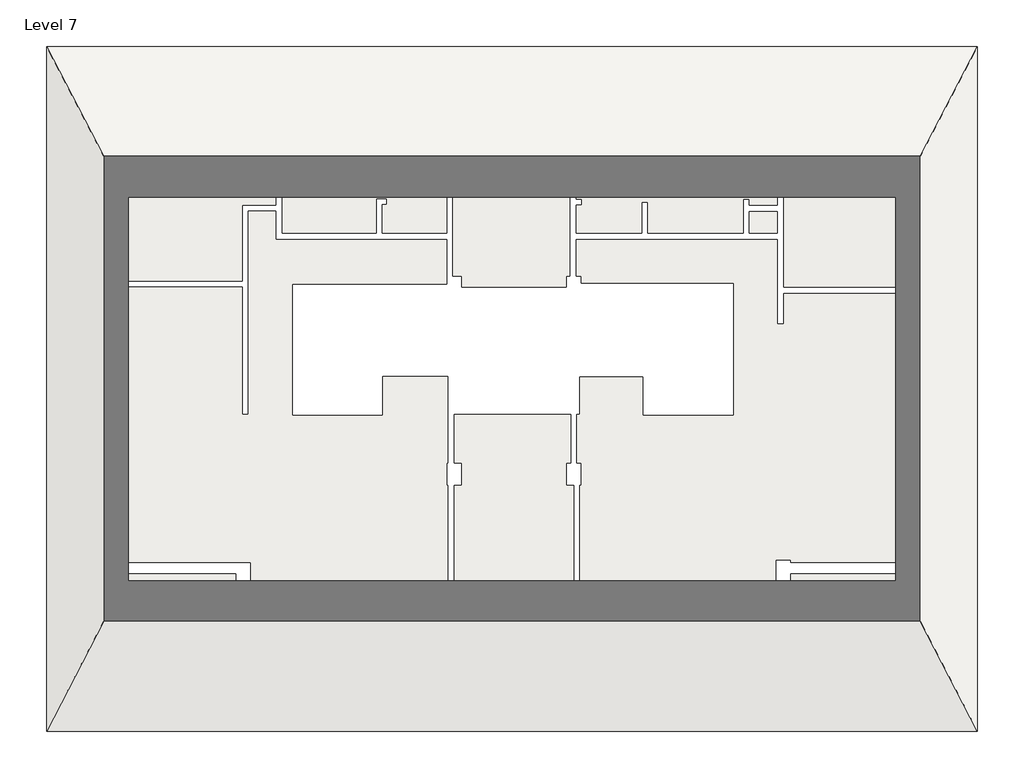
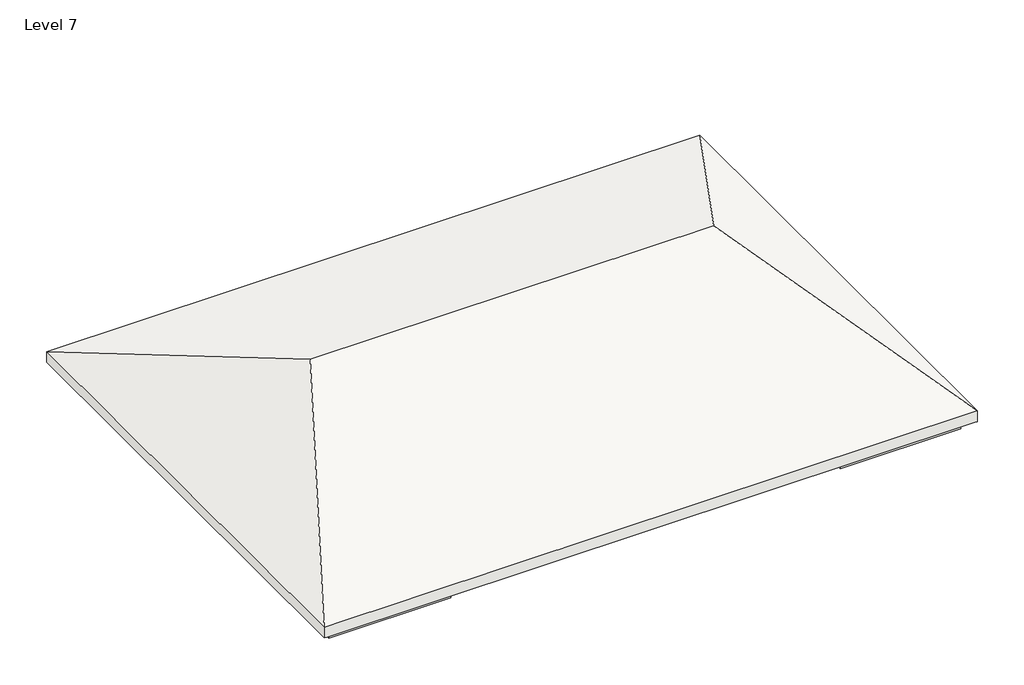
# One storey: 7 slabs, 1 roof.
"""IFC4 building model written with IfcOpenShell, lengths in millimetres."""

from ifc_helpers import new_model, si_unit, frame, origin, place, context, project, spatial, polyline, outline, extrude, faceted_brep, element, save

model = new_model("IFC4")

# Units and contexts
model_context = context("Model", 3, world=origin())
ifc_project = project(units=[si_unit("LENGTHUNIT", "METRE", prefix="MILLI")], contexts=[model_context])

# Site, building, storey
site = spatial("IfcSite", under=ifc_project)
building = spatial("IfcBuilding", under=site)
storey = spatial("IfcBuildingStorey", under=building, Name="Level 7", Elevation=12496.8)

# Roof
placement = place(None, origin())
element("IfcRoof", 1, ObjectType="roofing 1'", at=placement, inside=storey, context=model_context, shape_type="Brep", body=[
    faceted_brep([(9451.6503963, -918.8061634, 12496.8), (5824.1643827, -7900.2231861, 15217.4145102), (-5750.2606023, -7900.2231861, 15217.4145102), (-9377.7466158, -918.8061634, 12496.8), (-9377.7466158, -14881.6402089, 12496.8), (9451.6503963, -14881.6402089, 12496.8), (9523.4824202, -918.8061634, 12823.9259821), (-9449.5786397, -918.8061634, 12823.9259821), (-5822.0926261, -7900.2231861, 15544.5404923), (5895.9964066, -7900.2231861, 15544.5404923), (-9449.5786397, -14881.6402089, 12823.9259821), (9523.4824202, -14881.6402089, 12823.9259821), (-9449.5786397, -918.8061634, 12496.8), (9523.4824202, -918.8061634, 12496.8), (-9449.5786397, -14881.6402089, 12496.8), (9523.4824202, -14881.6402089, 12496.8)], [[[0, 1, 2, 3]], [[3, 2, 4]], [[4, 2, 1, 5]], [[1, 0, 5]], [[6, 7, 8, 9]], [[7, 10, 8]], [[10, 11, 9, 8]], [[6, 9, 11]], [[12, 7, 6, 13, 0, 3]], [[14, 10, 7, 12]], [[15, 11, 10, 14, 4, 5]], [[13, 6, 11, 15]], [[13, 15, 5, 0]], [[4, 14, 12, 3]]]),
])

# Slabs
element("IfcSlab", 2, ObjectType="flooring 1'", at=placement, inside=storey, context=model_context, shape_type="SweptSolid", body=[
    extrude(outline(polyline([(-8916.1786397, -11442.6620333), (-8916.1786397, -9867.8620333), (-8839.9786397, -9867.8620333), (-8839.9786397, -9410.6620333), (-8916.1786397, -9410.6620333), (-8916.1786397, -6057.8620333), (-8839.9786397, -6057.8620333), (-8839.9786397, -5829.2620333), (-5462.5175798, -5829.2620333), (-5462.5175798, -8420.0620333), (-5335.5175798, -8420.0620333), (-5335.5175798, -4280.3104011), (-4776.7175798, -4280.3104011), (-4776.7175798, -4855.8061634), (-1296.9175798, -4855.8061634), (-1296.9175798, -5600.6620333), (-1296.9175798, -5758.8942903), (-4442.5950401, -5758.8942903), (-4442.5950401, -8439.1120333), (-2601.0950401, -8439.1120333), (-2601.0950401, -7651.7120333), (-1271.5175798, -7651.7120333), (-1271.5175798, -9410.6620333), (-1296.9175798, -9410.6620333), (-1296.9175798, -9867.8620333), (-1271.5175798, -9867.8620333), (-1271.5175798, -12722.6402089), (-1779.5175798, -12722.6402089), (-1779.5175798, -14348.2402089), (-4548.1175798, -14348.2402089), (-4548.1175798, -14119.6402089), (-4852.9175798, -14119.6402089), (-4852.9175798, -14348.2402089), (-5360.9175798, -14348.2402089), (-5360.9175798, -11899.8620333), (-5284.7175798, -11899.8620333), (-5284.7175798, -11442.6620333), (-5589.5175798, -11442.6620333), (-8916.1786397, -11442.6620333)])), frame((0.0, 0.0, 12192.0), z_axis=(0.0, 0.0, 1.0), x_axis=(1.0, 0.0, 0.0)), (0.0, 0.0, 1.0), 304.8),
])
element("IfcSlab", 3, ObjectType="flooring 1'", at=placement, inside=storey, context=model_context, shape_type="SweptSolid", body=[
    extrude(outline(polyline([(5446.7824202, -4855.8061634), (5446.7824202, -6583.0061634), (5573.7824202, -6583.0061634), (5573.7824202, -5956.2620333), (8913.8824202, -5956.2620333), (8913.8824202, -6057.8620333), (8990.0824202, -6057.8620333), (8990.0824202, -9410.6620333), (8913.8824202, -9410.6620333), (8913.8824202, -9867.8620333), (8990.0824202, -9867.8620333), (8990.0824202, -11391.8620333), (8913.8824202, -11391.8620333), (8913.8824202, -11442.6620333), (5713.4824202, -11442.6620333), (5713.4824202, -11391.8620333), (5408.6824202, -11391.8620333), (5408.6824202, -11849.0620333), (5484.8824202, -11849.0620333), (5484.8824202, -14348.2402089), (4951.4824202, -14348.2402089), (4951.4824202, -14119.6402089), (4646.6824202, -14119.6402089), (4646.6824202, -14348.2402089), (1903.4824202, -14348.2402089), (1903.4824202, -12722.6402089), (1420.8824202, -12722.6402089), (1420.8824202, -9867.8620333), (1446.2824202, -9867.8620333), (1446.2824202, -9410.6620333), (1357.3824202, -9410.6620333), (1357.3824202, -8426.4120333), (1420.8824202, -8426.4120333), (1420.8824202, -7660.8890971), (2703.5824202, -7660.8890971), (2703.5824202, -8439.7691591), (4557.7824202, -8439.7691591), (4557.7824202, -5747.3691591), (1446.2824202, -5747.3691591), (1446.2824202, -5600.6620333), (1344.6824202, -5600.6620333), (1344.6824202, -4855.8061634), (5446.7824202, -4855.8061634)])), frame((0.0, 0.0, 12192.0), z_axis=(0.0, 0.0, 1.0), x_axis=(1.0, 0.0, 0.0)), (0.0, 0.0, 1.0), 304.8),
])
element("IfcSlab", 4, ObjectType="flooring 1'", at=placement, inside=storey, context=model_context, shape_type="SweptSolid", body=[
    extrude(outline(polyline([(-8839.9786397, -1680.8061634), (-8839.9786397, -1452.2061634), (-4852.9175798, -1452.2061634), (-4852.9175798, -1680.8061634), (-4776.7175798, -1680.8061634), (-4776.7175798, -4153.3104011), (-5462.5175798, -4153.3104011), (-5462.5175798, -5702.2620333), (-8839.9786397, -5702.2620333), (-8839.9786397, -5600.6620333), (-8916.1786397, -5600.6620333), (-8916.1786397, -1680.8061634), (-8839.9786397, -1680.8061634)])), frame((0.0, 0.0, 12192.0), z_axis=(0.0, 0.0, 1.0), x_axis=(1.0, 0.0, 0.0)), (0.0, 0.0, 1.0), 304.8),
    extrude(outline(polyline([(-2732.0175798, -4728.8061634), (-4649.7175798, -4728.8061634), (-4649.7175798, -1680.8061634), (-4548.1175798, -1680.8061634), (-4548.1175798, -1452.2061634), (-1296.9175798, -1452.2061634), (-1296.9175798, -4728.8061634), (-2605.0175798, -4728.8061634), (-2605.0175798, -4144.6061634), (-2516.1175798, -4144.6061634), (-2516.1175798, -4017.6061634), (-2732.0175798, -4017.6061634), (-2732.0175798, -4728.8061634)])), frame((0.0, 0.0, 12192.0), z_axis=(0.0, 0.0, 1.0), x_axis=(1.0, 0.0, 0.0)), (0.0, 0.0, 1.0), 304.8),
])
element("IfcSlab", 5, ObjectType="flooring 1'", at=placement, inside=storey, context=model_context, shape_type="SweptSolid", body=[
    extrude(outline(polyline([(4646.6824202, -1452.2061634), (4646.6824202, -1680.8061634), (4951.4824202, -1680.8061634), (4951.4824202, -1452.2061634), (5446.7824202, -1452.2061634), (5446.7824202, -4157.3061634), (4875.2824202, -4157.3061634), (4875.2824202, -4030.3061634), (4748.2824202, -4030.3061634), (4748.2824202, -4728.8061634), (2805.1824202, -4728.8061634), (2805.1824202, -4093.8061634), (2678.1824202, -4093.8061634), (2678.1824202, -4728.8061634), (1344.6824202, -4728.8061634), (1344.6824202, -4157.3061634), (1458.9824202, -4157.3061634), (1458.9824202, -4030.3061634), (1344.6824202, -4030.3061634), (1344.6824202, -1680.8061634), (1446.2824202, -1680.8061634), (1446.2824202, -1452.2061634), (4646.6824202, -1452.2061634)])), frame((0.0, 0.0, 12192.0), z_axis=(0.0, 0.0, 1.0), x_axis=(1.0, 0.0, 0.0)), (0.0, 0.0, 1.0), 304.8),
    extrude(outline(polyline([(5446.7824202, -4284.3061634), (5446.7824202, -4728.8061634), (4875.2824202, -4728.8061634), (4875.2824202, -4284.3061634), (5446.7824202, -4284.3061634)])), frame((0.0, 0.0, 12192.0), z_axis=(0.0, 0.0, 1.0), x_axis=(1.0, 0.0, 0.0)), (0.0, 0.0, 1.0), 304.8),
    extrude(outline(polyline([(8913.8824202, -5829.2620333), (5573.7824202, -5829.2620333), (5573.7824202, -1452.2061634), (8913.8824202, -1452.2061634), (8913.8824202, -1680.8061634), (8990.0824202, -1680.8061634), (8990.0824202, -5600.6620333), (8913.8824202, -5600.6620333), (8913.8824202, -5829.2620333)])), frame((0.0, 0.0, 12192.0), z_axis=(0.0, 0.0, 1.0), x_axis=(1.0, 0.0, 0.0)), (0.0, 0.0, 1.0), 304.8),
])
element("IfcSlab", 6, ObjectType="flooring 1'", at=placement, inside=storey, context=model_context, shape_type="SweptSolid", body=[
    extrude(outline(polyline([(1141.4824202, -1452.2061634), (1141.4824202, -1680.8061634), (1217.6824202, -1680.8061634), (1217.6824202, -5600.6620333), (1141.4824202, -5600.6620333), (1141.4824202, -5829.2620333), (-992.1175798, -5829.2620333), (-992.1175798, -5600.6620333), (-1169.9175798, -5600.6620333), (-1169.9175798, -1680.8061634), (-992.1175798, -1680.8061634), (-992.1175798, -1452.2061634), (1141.4824202, -1452.2061634)])), frame((0.0, 0.0, 12192.0), z_axis=(0.0, 0.0, 1.0), x_axis=(1.0, 0.0, 0.0)), (0.0, 0.0, 1.0), 304.8),
])
element("IfcSlab", 7, ObjectType="flooring 1'", at=placement, inside=storey, context=model_context, shape_type="SweptSolid", body=[
    extrude(outline(polyline([(1293.8824202, -12722.6402089), (-1144.5175798, -12722.6402089), (-1144.5175798, -9867.8620333), (-992.1175798, -9867.8620333), (-992.1175798, -9410.6620333), (-1144.5175798, -9410.6620333), (-1144.5175798, -8426.4120333), (1230.3824202, -8426.4120333), (1230.3824202, -9410.6620333), (1141.4824202, -9410.6620333), (1141.4824202, -9867.8620333), (1293.8824202, -9867.8620333), (1293.8824202, -12722.6402089)])), frame((0.0, 0.0, 12192.0), z_axis=(0.0, 0.0, 1.0), x_axis=(1.0, 0.0, 0.0)), (0.0, 0.0, 1.0), 304.8),
])
element("IfcSlab", 8, ObjectType="flooring 1'", at=placement, inside=storey, context=model_context, shape_type="SweptSolid", body=[
    extrude(outline(polyline([(-5589.5175798, -11671.2620333), (-5589.5175798, -14576.8402089), (-9144.7786397, -14576.8402089), (-9144.7786397, -11671.2620333), (-5589.5175798, -11671.2620333)])), frame((0.0, 0.0, 12192.0), z_axis=(0.0, 0.0, 1.0), x_axis=(1.0, 0.0, 0.0)), (0.0, 0.0, 1.0), 304.8),
    extrude(outline(polyline([(9218.6824202, -11671.2620333), (9218.6824202, -14576.8402089), (5713.4824202, -14576.8402089), (5713.4824202, -11671.2620333), (9218.6824202, -11671.2620333)])), frame((0.0, 0.0, 12192.0), z_axis=(0.0, 0.0, 1.0), x_axis=(1.0, 0.0, 0.0)), (0.0, 0.0, 1.0), 304.8),
])

save(model, "model.ifc")

# Revit data of these elements
# Type "roofing 1'"
#   Assembly Code = "B1020"
#   Layers, outside or top first: 1' - 0" "roofing 1'" (function 1)
# Type "flooring 1'"
#   Assembly Code = "B1010"
#   Function = 0
#   Layers, outside or top first: 1' - 0" "FL_MARBLE WHITE" (function 1)
# Element 1 (IfcRoof, "roofing 1'")
#   built-in parameter 1001705 = 50.9991 (stored number, unit not read)
#   built-in parameter 1001710 = 33615
#   Phase Created = New Construction
#   Materials on its faces: "roofing 1'"
# Element 2 (IfcSlab, "flooring 1'")
#   built-in parameter 1001955 = 3.14159 (stored number, unit not read)
#   Height Offset From Level = 0' - 0"
#   Phase Created = New Construction
#   Materials on its faces: "FL_MARBLE WHITE"
# Elements 3, 5, 6, 7, 8 (IfcSlab, "flooring 1'")
#   Height Offset From Level = 0' - 0"
#   Phase Created = New Construction
#   Materials on its faces: "FL_MARBLE WHITE"
# Element 4 (IfcSlab, "flooring 1'")
#   built-in parameter 1001955 = -1.5708 (stored number, unit not read)
#   Height Offset From Level = 0' - 0"
#   Phase Created = New Construction
#   Materials on its faces: "FL_MARBLE WHITE"
# Materials
#   "roofing 1'": class "Generic", colour RGB 120 120 120, transparency 0, Cost = 0
#   "FL_MARBLE WHITE": class "Generic", colour RGB 120 120 120, transparency 0, Cost = 0
